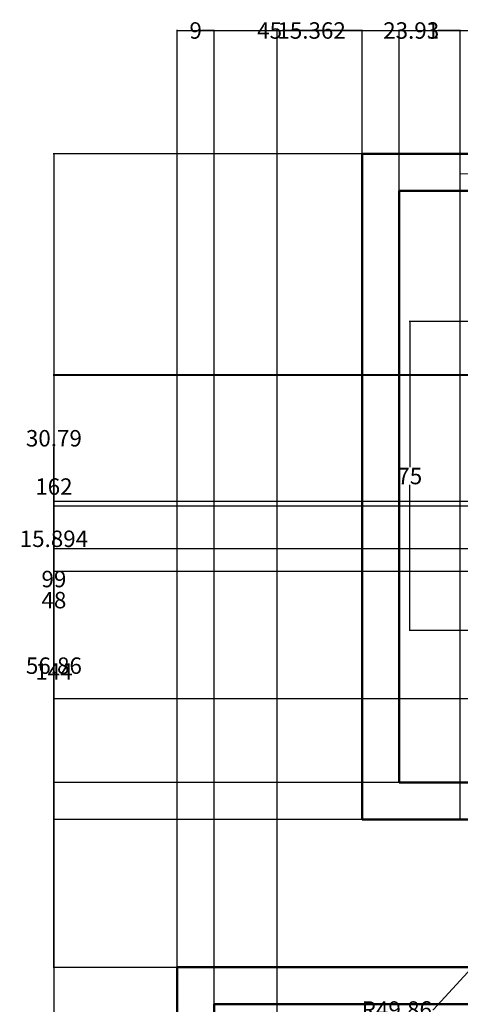
# Model space of a CAD drawing. Units: inches. Extents: x 1454 to 2136, y 626 to 1213.
# Tile 5 of 23: x 1454 to 1561, y 973 to 1213. Entities that reach past the tile are written whole.
import ezdxf

# ---------------------------------------------------------------- set-up
doc = ezdxf.new("R2010")
doc.units = ezdxf.units.IN
doc.header["$MEASUREMENT"] = 0
for name, color, linetype, lineweight in [('A-ANNO-DIMS', 2, 'Continuous', 18), ('A-FURN-PATT', 252, 'Continuous', 13), ('A-GLAZ', 4, 'Continuous', 18), ('A-WALL', 7, 'Continuous', 50)]:
    doc.layers.add(name, color=color, linetype=linetype, lineweight=lineweight)
doc.styles.get("Standard").update_dxf_attribs({"font": 'arial.ttf'})
doc.dimstyles.get("Standard").update_dxf_attribs({"dimtxt": 4, "dimasz": 0.18, "dimexe": 0.18, "dimexo": 0.0625, "dimgap": 0.09, "dimtad": 0, "dimtih": 1, "dimtoh": 1, "dimdec": 0, "dimrnd": 6, "dimzin": 0, "dimdsep": 46, "dimlunit": 3, "dimtxsty": 'Standard', "dimcen": 0.09, "dimadec": 0, "dimazin": 0, "dimtfac": 1, "dimtdec": 0, "dimtofl": 0, "dimtmove": 0, "dimatfit": 3, "dimfxl": 1, "dimtolj": 1, "dimtzin": 0, "dimarcsym": 0})

# ---------------------------------------------------------------- blocks, each defined once
blk = doc.blocks.new('WIN-34_84')
blk.add_line((34.84, 4.31), (0, 4.31))
blk.add_lwpolyline([(34.84, 0), (0, 0), (0, 9), (34.84, 9)], close=True)
blk = doc.blocks.new('*D24')
at = {"layer": 'A-ANNO-DIMS', "color": 0, "lineweight": -2, "transparency": 16777216}
for p, q in [((1571.61, 1139.47), (1548.99, 1139.47)), ((1549.17, 1139.29), (1549.17, 1103.97)), ((1549.17, 1064.4), (1549.17, 1099.72)), ((1571.61, 1064.22), (1548.99, 1064.22))]:
    blk.add_line(p, q, dxfattribs=at)
at = {"layer": 'A-ANNO-DIMS', "color": 0, "transparency": 16777216}
for points in [[(1549.14, 1139.29), (1549.2, 1139.29), (1549.17, 1139.47)], [(1549.14, 1064.4), (1549.2, 1064.4), (1549.17, 1064.22)]]:
    blk.add_solid(points, dxfattribs=at)
at = {"layer": 'Defpoints', "color": 0, "transparency": 16777216}
for p in [(1549.17, 1139.47), (1571.67, 1139.47), (1571.67, 1064.22)]:
    blk.add_point(p, dxfattribs=at)
at = {"layer": 'A-ANNO-DIMS', "color": 0, "transparency": 16777216, "insert": (1549.17, 1101.85), "char_height": 4, "attachment_point": 5}
blk.add_mtext('\\A1;75', dxfattribs=at)
blk = doc.blocks.new('*D28')
at = {"layer": 'A-ANNO-DIMS', "color": 0, "lineweight": -2, "transparency": 16777216}
for p, q in [((1537.49, 1180.28), (1462.37, 1180.28)), ((1462.55, 1180.1), (1462.55, 921.41)), ((1462.55, 658.46), (1462.55, 917.15)), ((1492.49, 658.28), (1462.37, 658.28))]:
    blk.add_line(p, q, dxfattribs=at)
at = {"layer": 'A-ANNO-DIMS', "color": 0, "transparency": 16777216}
for points in [[(1462.52, 1180.1), (1462.58, 1180.1), (1462.55, 1180.28)], [(1462.52, 658.46), (1462.58, 658.46), (1462.55, 658.28)]]:
    blk.add_solid(points, dxfattribs=at)
at = {"layer": 'Defpoints', "color": 0, "transparency": 16777216}
for p in [(1462.55, 1180.28), (1537.56, 1180.28), (1492.56, 658.28)]:
    blk.add_point(p, dxfattribs=at)
at = {"layer": 'A-ANNO-DIMS', "color": 0, "transparency": 16777216, "insert": (1462.55, 919.28), "char_height": 4, "attachment_point": 5}
blk.add_mtext('\\A1;522', dxfattribs=at)
blk = doc.blocks.new('*D29')
at = {"layer": 'A-ANNO-DIMS', "color": 0, "lineweight": -2, "transparency": 16777216}
for p, q in [((1546.56, 1171.34), (1546.56, 1210.46)), ((1546.74, 1210.28), (1644.02, 1210.28)), ((1750.38, 1210.28), (1653.09, 1210.28)), ((1750.56, 1171.34), (1750.56, 1210.46))]:
    blk.add_line(p, q, dxfattribs=at)
at = {"layer": 'A-ANNO-DIMS', "color": 0, "transparency": 16777216}
for points in [[(1546.74, 1210.31), (1546.74, 1210.25), (1546.56, 1210.28)], [(1750.38, 1210.31), (1750.38, 1210.25), (1750.56, 1210.28)]]:
    blk.add_solid(points, dxfattribs=at)
at = {"layer": 'Defpoints', "color": 0, "transparency": 16777216}
for p in [(1750.56, 1210.28), (1546.56, 1171.28), (1750.56, 1171.28)]:
    blk.add_point(p, dxfattribs=at)
at = {"layer": 'A-ANNO-DIMS', "color": 0, "transparency": 16777216, "insert": (1648.56, 1210.28), "char_height": 4, "attachment_point": 5}
blk.add_mtext('\\A1;204', dxfattribs=at)
blk = doc.blocks.new('*D30')
at = {"layer": 'A-ANNO-DIMS', "color": 0, "lineweight": -2, "transparency": 16777216}
for p, q in [((1537.49, 1180.28), (1462.37, 1180.28)), ((1462.55, 1180.1), (1462.55, 1101.41)), ((1462.55, 1018.46), (1462.55, 1097.15)), ((1537.49, 1018.28), (1462.37, 1018.28))]:
    blk.add_line(p, q, dxfattribs=at)
at = {"layer": 'A-ANNO-DIMS', "color": 0, "transparency": 16777216}
for points in [[(1462.52, 1180.1), (1462.58, 1180.1), (1462.55, 1180.28)], [(1462.52, 1018.46), (1462.58, 1018.46), (1462.55, 1018.28)]]:
    blk.add_solid(points, dxfattribs=at)
at = {"layer": 'Defpoints', "color": 0, "transparency": 16777216}
for p in [(1462.55, 1180.28), (1537.56, 1180.28), (1537.56, 1018.28)]:
    blk.add_point(p, dxfattribs=at)
at = {"layer": 'A-ANNO-DIMS', "color": 0, "transparency": 16777216, "insert": (1462.55, 1099.28), "char_height": 4, "attachment_point": 5}
blk.add_mtext('\\A1;162', dxfattribs=at)
blk = doc.blocks.new('*D33')
at = {"layer": 'A-ANNO-DIMS', "color": 0, "lineweight": -2, "transparency": 16777216}
for p, q in [((2032.49, 1126.28), (1462.37, 1126.28)), ((1462.55, 1126.1), (1462.55, 1056.38)), ((1462.55, 982.46), (1462.55, 1052.18)), ((2032.49, 982.28), (1462.37, 982.28))]:
    blk.add_line(p, q, dxfattribs=at)
at = {"layer": 'A-ANNO-DIMS', "color": 0, "transparency": 16777216}
for points in [[(1462.52, 1126.1), (1462.58, 1126.1), (1462.55, 1126.28)], [(1462.52, 982.46), (1462.58, 982.46), (1462.55, 982.28)]]:
    blk.add_solid(points, dxfattribs=at)
at = {"layer": 'Defpoints', "color": 0, "transparency": 16777216}
for p in [(1462.55, 1126.28), (2032.56, 1126.28), (2032.56, 982.28)]:
    blk.add_point(p, dxfattribs=at)
at = {"layer": 'A-ANNO-DIMS', "color": 0, "transparency": 16777216, "insert": (1462.55, 1054.28), "char_height": 4, "attachment_point": 5}
blk.add_mtext('\\A1;144', dxfattribs=at)
blk = doc.blocks.new('*D39')
at = {"layer": 'A-ANNO-DIMS', "color": 0, "lineweight": -2, "transparency": 16777216}
for p, q in [((1492.56, 982.34), (1492.56, 1210.46)), ((1492.74, 1210.28), (1512.01, 1210.28)), ((1537.38, 1210.28), (1518.11, 1210.28)), ((1537.56, 1018.34), (1537.56, 1210.46))]:
    blk.add_line(p, q, dxfattribs=at)
at = {"layer": 'A-ANNO-DIMS', "color": 0, "transparency": 16777216}
for points in [[(1492.74, 1210.31), (1492.74, 1210.25), (1492.56, 1210.28)], [(1537.38, 1210.31), (1537.38, 1210.25), (1537.56, 1210.28)]]:
    blk.add_solid(points, dxfattribs=at)
at = {"layer": 'Defpoints', "color": 0, "transparency": 16777216}
for p in [(1537.56, 1210.28), (1537.56, 1018.28), (1492.56, 982.28)]:
    blk.add_point(p, dxfattribs=at)
at = {"layer": 'A-ANNO-DIMS', "color": 0, "transparency": 16777216, "insert": (1515.06, 1210.28), "char_height": 4, "attachment_point": 5}
blk.add_mtext('\\A1;45', dxfattribs=at)
blk = doc.blocks.new('*D40')
at = {"layer": 'A-ANNO-DIMS', "color": 0, "lineweight": -2, "transparency": 16777216}
for p, q in [((1501.56, 877.34), (1501.56, 1210.46)), ((1501.74, 1210.28), (1569.24, 1210.28)), ((1645.38, 1210.28), (1577.87, 1210.28)), ((1645.56, 877.34), (1645.56, 1210.46))]:
    blk.add_line(p, q, dxfattribs=at)
at = {"layer": 'A-ANNO-DIMS', "color": 0, "transparency": 16777216}
for points in [[(1501.74, 1210.31), (1501.74, 1210.25), (1501.56, 1210.28)], [(1645.38, 1210.31), (1645.38, 1210.25), (1645.56, 1210.28)]]:
    blk.add_solid(points, dxfattribs=at)
at = {"layer": 'Defpoints', "color": 0, "transparency": 16777216}
for p in [(1645.56, 1210.28), (1501.56, 877.28), (1645.56, 877.28)]:
    blk.add_point(p, dxfattribs=at)
at = {"layer": 'A-ANNO-DIMS', "color": 0, "transparency": 16777216, "insert": (1573.56, 1210.28), "char_height": 4, "attachment_point": 5}
blk.add_mtext('\\A1;144', dxfattribs=at)
blk = doc.blocks.new('*D49')
at = {"layer": 'A-ANNO-DIMS', "color": 0, "lineweight": -2, "transparency": 16777216}
for p, q in [((1537.56, 1180.34), (1537.56, 1210.46)), ((1537.74, 1210.28), (1543.02, 1210.28)), ((1561.28, 1210.28), (1556, 1210.28)), ((1561.46, 1180.17), (1561.46, 1210.46))]:
    blk.add_line(p, q, dxfattribs=at)
at = {"layer": 'A-ANNO-DIMS', "color": 0, "transparency": 16777216}
for points in [[(1537.74, 1210.31), (1537.74, 1210.25), (1537.56, 1210.28)], [(1561.28, 1210.31), (1561.28, 1210.25), (1561.46, 1210.28)]]:
    blk.add_solid(points, dxfattribs=at)
at = {"layer": 'Defpoints', "color": 0, "transparency": 16777216}
for p in [(1561.46, 1210.28), (1537.56, 1180.28), (1561.46, 1180.1)]:
    blk.add_point(p, dxfattribs=at)
at = {"layer": 'A-ANNO-DIMS', "color": 0, "transparency": 16777216, "insert": (1549.51, 1210.28), "char_height": 4, "attachment_point": 5}
blk.add_mtext('\\A1;23.91', dxfattribs=at)
blk = doc.blocks.new('*D54')
at = {"layer": 'A-ANNO-DIMS', "color": 0, "lineweight": -2, "transparency": 16777216}
for p, q in [((1879.49, 1126.28), (1462.37, 1126.28)), ((1462.55, 1126.1), (1462.55, 1078.91)), ((1462.55, 1027.46), (1462.55, 1074.65)), ((1879.49, 1027.28), (1462.37, 1027.28))]:
    blk.add_line(p, q, dxfattribs=at)
at = {"layer": 'A-ANNO-DIMS', "color": 0, "transparency": 16777216}
for points in [[(1462.52, 1126.1), (1462.58, 1126.1), (1462.55, 1126.28)], [(1462.52, 1027.46), (1462.58, 1027.46), (1462.55, 1027.28)]]:
    blk.add_solid(points, dxfattribs=at)
at = {"layer": 'Defpoints', "color": 0, "transparency": 16777216}
for p in [(1879.56, 1126.28), (1462.55, 1027.28), (1879.56, 1027.28)]:
    blk.add_point(p, dxfattribs=at)
at = {"layer": 'A-ANNO-DIMS', "color": 0, "transparency": 16777216, "insert": (1462.55, 1076.78), "char_height": 4, "attachment_point": 5}
blk.add_mtext('\\A1;99', dxfattribs=at)
blk = doc.blocks.new('*D55')
at = {"layer": 'A-ANNO-DIMS', "color": 0, "lineweight": -2, "transparency": 16777216}
for p, q in [((1537.56, 1018.34), (1537.56, 1210.46)), ((1537.74, 1210.28), (1542.65, 1210.28)), ((1561.3, 1210.28), (1556.39, 1210.28)), ((1561.48, 1018.34), (1561.48, 1210.46))]:
    blk.add_line(p, q, dxfattribs=at)
at = {"layer": 'A-ANNO-DIMS', "color": 0, "transparency": 16777216}
for points in [[(1537.74, 1210.31), (1537.74, 1210.25), (1537.56, 1210.28)], [(1561.3, 1210.31), (1561.3, 1210.25), (1561.48, 1210.28)]]:
    blk.add_solid(points, dxfattribs=at)
at = {"layer": 'Defpoints', "color": 0, "transparency": 16777216}
for p in [(1561.48, 1210.28), (1537.56, 1018.28), (1561.48, 1018.28)]:
    blk.add_point(p, dxfattribs=at)
at = {"layer": 'A-ANNO-DIMS', "color": 0, "transparency": 16777216, "insert": (1549.52, 1210.28), "char_height": 4, "attachment_point": 5}
blk.add_mtext('\\A1;23.93', dxfattribs=at)
blk = doc.blocks.new('*D70')
at = {"layer": 'A-ANNO-DIMS', "color": 0, "lineweight": -2, "transparency": 16777216}
for p, q in [((1811.17, 1094.52), (1462.37, 1094.52)), ((1462.55, 1094.34), (1462.55, 1088.71)), ((1462.55, 1078.81), (1462.55, 1084.45)), ((1811.17, 1078.63), (1462.37, 1078.63))]:
    blk.add_line(p, q, dxfattribs=at)
at = {"layer": 'A-ANNO-DIMS', "color": 0, "transparency": 16777216}
for points in [[(1462.52, 1094.34), (1462.58, 1094.34), (1462.55, 1094.52)], [(1462.52, 1078.81), (1462.58, 1078.81), (1462.55, 1078.63)]]:
    blk.add_solid(points, dxfattribs=at)
at = {"layer": 'Defpoints', "color": 0, "transparency": 16777216}
for p in [(1462.55, 1094.52), (1811.23, 1094.52), (1811.23, 1078.63)]:
    blk.add_point(p, dxfattribs=at)
at = {"layer": 'A-ANNO-DIMS', "color": 0, "transparency": 16777216, "insert": (1462.55, 1086.58), "char_height": 4, "attachment_point": 5}
blk.add_mtext('\\A1;15.894', dxfattribs=at)
blk = doc.blocks.new('*D73')
at = {"layer": 'A-ANNO-DIMS', "color": 0, "lineweight": -2, "transparency": 16777216}
for p, q in [((1985.1, 1126.44), (1462.37, 1126.44)), ((1462.55, 1126.26), (1462.55, 1113.18)), ((1462.55, 1095.83), (1462.55, 1108.91)), ((1966.64, 1095.65), (1462.37, 1095.65))]:
    blk.add_line(p, q, dxfattribs=at)
at = {"layer": 'A-ANNO-DIMS', "color": 0, "transparency": 16777216}
for points in [[(1462.52, 1126.26), (1462.58, 1126.26), (1462.55, 1126.44)], [(1462.52, 1095.83), (1462.58, 1095.83), (1462.55, 1095.65)]]:
    blk.add_solid(points, dxfattribs=at)
at = {"layer": 'Defpoints', "color": 0, "transparency": 16777216}
for p in [(1985.16, 1126.44), (1462.55, 1095.65), (1966.71, 1095.65)]:
    blk.add_point(p, dxfattribs=at)
at = {"layer": 'A-ANNO-DIMS', "color": 0, "transparency": 16777216, "insert": (1462.55, 1111.04), "char_height": 4, "attachment_point": 5}
blk.add_mtext('\\A1;30.79', dxfattribs=at)
blk = doc.blocks.new('*D76')
at = {"layer": 'A-ANNO-DIMS', "color": 0, "lineweight": -2, "transparency": 16777216}
for p, q in [((1962.64, 1095.65), (1462.37, 1095.65)), ((1462.55, 1095.47), (1462.55, 1073.78)), ((1462.55, 1047.83), (1462.55, 1069.52)), ((1914.64, 1047.65), (1462.37, 1047.65))]:
    blk.add_line(p, q, dxfattribs=at)
at = {"layer": 'A-ANNO-DIMS', "color": 0, "transparency": 16777216}
for points in [[(1462.52, 1095.47), (1462.58, 1095.47), (1462.55, 1095.65)], [(1462.52, 1047.83), (1462.58, 1047.83), (1462.55, 1047.65)]]:
    blk.add_solid(points, dxfattribs=at)
at = {"layer": 'Defpoints', "color": 0, "transparency": 16777216}
for p in [(1962.71, 1095.65), (1462.55, 1047.65), (1914.71, 1047.65)]:
    blk.add_point(p, dxfattribs=at)
at = {"layer": 'A-ANNO-DIMS', "color": 0, "transparency": 16777216, "insert": (1462.55, 1071.65), "char_height": 4, "attachment_point": 5}
blk.add_mtext('\\A1;48', dxfattribs=at)
blk = doc.blocks.new('*D79')
at = {"layer": 'A-ANNO-DIMS', "color": 0, "lineweight": -2, "transparency": 16777216}
for p, q in [((1501.56, 973.34), (1501.56, 1210.46)), ((1501.74, 1210.28), (1516.74, 1210.28)), ((1516.92, 962.3), (1516.92, 1210.46)), ((1516.92, 1210.28), (1517.1, 1210.28))]:
    blk.add_line(p, q, dxfattribs=at)
at = {"layer": 'A-ANNO-DIMS', "color": 0, "transparency": 16777216}
for points in [[(1501.74, 1210.31), (1501.74, 1210.25), (1501.56, 1210.28)], [(1516.74, 1210.31), (1516.74, 1210.25), (1516.92, 1210.28)]]:
    blk.add_solid(points, dxfattribs=at)
at = {"layer": 'Defpoints', "color": 0, "transparency": 16777216}
for p in [(1516.92, 1210.28), (1501.56, 973.28), (1516.92, 962.24)]:
    blk.add_point(p, dxfattribs=at)
at = {"layer": 'A-ANNO-DIMS', "color": 0, "transparency": 16777216, "insert": (1525.28, 1210.28), "char_height": 4, "attachment_point": 5}
blk.add_mtext('\\A1;15.362', dxfattribs=at)
blk = doc.blocks.new('*D82')
at = {"layer": 'A-ANNO-DIMS', "color": 0, "lineweight": -2, "transparency": 16777216}
for p, q in [((1697.82, 1084.13), (1462.37, 1084.13)), ((1462.55, 1083.95), (1462.55, 1057.83)), ((1462.55, 1027.45), (1462.55, 1053.57)), ((1704.25, 1027.27), (1462.37, 1027.27))]:
    blk.add_line(p, q, dxfattribs=at)
at = {"layer": 'A-ANNO-DIMS', "color": 0, "transparency": 16777216}
for points in [[(1462.52, 1083.95), (1462.58, 1083.95), (1462.55, 1084.13)], [(1462.52, 1027.45), (1462.58, 1027.45), (1462.55, 1027.27)]]:
    blk.add_solid(points, dxfattribs=at)
at = {"layer": 'Defpoints', "color": 0, "transparency": 16777216}
for p in [(1462.55, 1084.13), (1697.88, 1084.13), (1704.31, 1027.27)]:
    blk.add_point(p, dxfattribs=at)
at = {"layer": 'A-ANNO-DIMS', "color": 0, "transparency": 16777216, "insert": (1462.55, 1055.7), "char_height": 4, "attachment_point": 5}
blk.add_mtext('\\A1;56.86', dxfattribs=at)
blk = doc.blocks.new('*D88')
at = {"layer": 'A-ANNO-DIMS', "color": 0, "lineweight": -2, "transparency": 16777216}
for p, q in [((1492.56, 658.34), (1492.56, 1210.46)), ((1492.74, 1210.28), (1495.65, 1210.28)), ((1501.38, 1210.28), (1498.46, 1210.28)), ((1501.56, 667.34), (1501.56, 1210.46))]:
    blk.add_line(p, q, dxfattribs=at)
at = {"layer": 'A-ANNO-DIMS', "color": 0, "transparency": 16777216}
for points in [[(1492.74, 1210.31), (1492.74, 1210.25), (1492.56, 1210.28)], [(1501.38, 1210.31), (1501.38, 1210.25), (1501.56, 1210.28)]]:
    blk.add_solid(points, dxfattribs=at)
at = {"layer": 'Defpoints', "color": 0, "transparency": 16777216}
for p in [(1501.56, 1210.28), (1501.56, 667.28), (1492.56, 658.28)]:
    blk.add_point(p, dxfattribs=at)
at = {"layer": 'A-ANNO-DIMS', "color": 0, "transparency": 16777216, "insert": (1497.06, 1210.28), "char_height": 4, "attachment_point": 5}
blk.add_mtext('\\A1;9', dxfattribs=at)
blk = doc.blocks.new('*D92')
at = {"layer": 'A-ANNO-DIMS', "color": 0, "lineweight": -2, "transparency": 16777216}
for p, q in [((1608.77, 1030.83), (1608.95, 1030.83)), ((1608.86, 1030.74), (1608.86, 1030.92)), ((1554.95, 972.02), (1575.05, 993.94)), ((1554.77, 972.02), (1554.95, 972.02))]:
    blk.add_line(p, q, dxfattribs=at)
at = {"layer": 'A-ANNO-DIMS', "color": 0, "transparency": 16777216}
blk.add_solid([(1575.02, 993.96), (1575.07, 993.92), (1575.17, 994.07)], dxfattribs=at)
at = {"layer": 'Defpoints', "color": 0, "transparency": 16777216}
for p in [(1608.86, 1030.83), (1575.17, 994.07)]:
    blk.add_point(p, dxfattribs=at)
at = {"layer": 'A-ANNO-DIMS', "color": 0, "transparency": 16777216, "insert": (1546.02, 972.02), "char_height": 4, "attachment_point": 5}
blk.add_mtext('\\A1;R49.86', dxfattribs=at)

msp = doc.modelspace()

# ---------------------------------------------------------------- hatches: boundary and pattern name
at = {"layer": 'A-FURN-PATT'}
h = msp.add_hatch(dxfattribs=at)
h.set_pattern_fill('ESCHER', color=256)
h.paths.add_polyline_path([(1511.3761, 923.7174, 1), (1525.379, 923.7174, 1)])
h.paths.add_polyline_path([(1525.379, 816.0542, 1), (1511.3761, 816.0542, 1)])
h.paths.add_polyline_path([(1525.379, 712.7345, 1), (1511.3761, 712.7345, 1)])
h.paths.add_polyline_path([(2070.5057, 794.3402, 1), (2056.5027, 794.3402, 1)])
h.paths.add_polyline_path([(2005.868, 1014.5578, 1), (1991.8651, 1014.5578, 1)])
h.paths.add_polyline_path([(1994.0647, 1066.7584, 1), (2008.0677, 1066.7584, 1)])
h.paths.add_polyline_path([(1919.5492, 1065.3848, 1), (1933.5521, 1065.3848, 1)])
h.paths.add_polyline_path([(1936.8517, 1013.7336, 1), (1922.8488, 1013.7336, 1)])
h.paths.add_polyline_path([(1824.6062, 1109.1557, 1), (1838.6091, 1109.1557, 1)])

# ---------------------------------------------------------------- linework, layer by layer
at = {"layer": 'A-WALL'}
for p, q in [((1759.5563, 1180.2825), (1537.5563, 1180.2825)), ((1537.5563, 1180.2825), (1537.5563, 1018.2825)), ((1750.5563, 1171.2825), (1546.5563, 1171.2825)), ((1546.5563, 1171.2825), (1546.5563, 1027.2825)), ((1750.5563, 1027.2825), (1546.5563, 1027.2825)), ((1843.5563, 1018.2825), (1537.5563, 1018.2825)), ((1492.5563, 982.2825), (1492.5563, 700.2825)), ((1654.5563, 982.2825), (1492.5563, 982.2825)), ((1501.5563, 973.2825), (1501.5563, 877.2825)), ((1645.5563, 973.2825), (1501.5563, 973.2825))]:
    msp.add_line(p, q, dxfattribs=at)

# ---------------------------------------------------------------- block references
at = {"layer": 'A-GLAZ'}
msp.add_blockref('WIN-34_84', (1561.4646, 1171.1038), dxfattribs=at)

# ---------------------------------------------------------------- dimensions: what is measured, and where the dimension line sits
at = {"layer": 'A-ANNO-DIMS'}
for base, p1, p2, override, picture, middle in [((1537.5563, 1210.2845), (1492.5563, 982.2825), (1537.5563, 1018.2825), {"dimdec": 0, "dimlfac": 1, "dimrnd": 0, "dimzin": 0, "dimdsep": 46, "dimlunit": 2}, '*D39', (1515.0563, 1210.2845)), ((1501.5563, 1210.2845), (1492.5563, 658.2825), (1501.5563, 667.2825), {"dimdec": 0, "dimlfac": 1, "dimrnd": 0, "dimzin": 0, "dimdsep": 46, "dimlunit": 2}, '*D88', (1497.0563, 1210.2845)), ((1645.5563, 1210.2845), (1501.5563, 877.2825), (1645.5563, 877.2825), {"dimdec": 0, "dimlfac": 1, "dimrnd": 0, "dimzin": 0, "dimdsep": 46, "dimlunit": 2}, '*D40', (1573.5563, 1210.2845)), ((1516.9185, 1210.2845), (1501.5563, 973.2825), (1516.9185, 962.2419), {"dimdec": 3, "dimlfac": 1, "dimrnd": 0, "dimzin": 0, "dimdsep": 46, "dimlunit": 2}, '*D79', (1525.2826, 1210.2845)), ((1561.4646, 1210.2845), (1537.5563, 1180.2825), (1561.4646, 1180.1038), {"dimdec": 2, "dimlfac": 1, "dimrnd": 0, "dimzin": 0, "dimdsep": 46, "dimlunit": 2}, '*D49', (1549.5105, 1210.2845)), ((1561.4844, 1210.2845), (1537.5563, 1018.2825), (1561.4844, 1018.2825), {"dimdec": 2, "dimlfac": 1, "dimrnd": 0, "dimzin": 0, "dimdsep": 46, "dimlunit": 2}, '*D55', (1549.5203, 1210.2845)), ((1750.5563, 1210.2845), (1546.5563, 1171.2825), (1750.5563, 1171.2825), {"dimdec": 0, "dimlfac": 1, "dimrnd": 0, "dimzin": 0, "dimdsep": 46, "dimlunit": 2}, '*D29', (1648.5563, 1210.2845))]:
    dim = msp.add_linear_dim(base=base, p1=p1, p2=p2, dimstyle='Standard', override=override, dxfattribs=at)
    dim.commit()
    dim.dimension.update_dxf_attribs({"geometry": picture, "text_midpoint": middle})
for base, p1, p2, override, picture, middle in [((1462.5543, 1180.2825), (1492.5563, 658.2825), (1537.5563, 1180.2825), {"dimdec": 0, "dimlfac": 1, "dimrnd": 0, "dimzin": 0, "dimdsep": 46, "dimlunit": 2}, '*D28', (1462.5543, 919.2825)), ((1462.5543, 1180.2825), (1537.5563, 1018.2825), (1537.5563, 1180.2825), {"dimdec": 0, "dimlfac": 1, "dimrnd": 0, "dimzin": 0, "dimdsep": 46, "dimlunit": 2}, '*D30', (1462.5543, 1099.2825)), ((1549.1663, 1139.4691), (1571.674, 1064.221), (1571.674, 1139.4691), {"dimdec": 0, "dimlfac": 1, "dimrnd": 0, "dimzin": 0, "dimdsep": 46, "dimlunit": 2}, '*D24', (1549.1663, 1101.8451)), ((1462.5543, 1095.6495), (1985.1581, 1126.439), (1966.7068, 1095.6495), {"dimdec": 2, "dimlfac": 1, "dimrnd": 0, "dimzin": 0, "dimdsep": 46, "dimlunit": 2}, '*D73', (1462.5543, 1111.0443)), ((1462.5543, 1126.2825), (2032.5563, 982.2825), (2032.5563, 1126.2825), {"dimdec": 0, "dimlfac": 1, "dimrnd": 0, "dimzin": 0, "dimdsep": 46, "dimlunit": 2}, '*D33', (1462.5543, 1054.2825)), ((1462.5543, 1027.2825), (1879.5563, 1126.2825), (1879.5563, 1027.2825), {"dimdec": 0, "dimlfac": 1, "dimrnd": 0, "dimzin": 0, "dimdsep": 46, "dimlunit": 2}, '*D54', (1462.5543, 1076.7825)), ((1462.5543, 1047.6495), (1962.7068, 1095.6495), (1914.7068, 1047.6495), {"dimdec": 0, "dimlfac": 1, "dimrnd": 0, "dimzin": 0, "dimdsep": 46, "dimlunit": 2}, '*D76', (1462.5543, 1071.6495)), ((1462.5543, 1094.5248), (1811.2288, 1078.6305), (1811.2288, 1094.5248), {"dimdec": 3, "dimlfac": 1, "dimrnd": 0, "dimzin": 0, "dimdsep": 46, "dimlunit": 2}, '*D70', (1462.5543, 1086.5777)), ((1462.5543, 1084.1285), (1704.308, 1027.2667), (1697.8807, 1084.1285), {"dimdec": 2, "dimlfac": 1, "dimrnd": 0, "dimzin": 0, "dimdsep": 46, "dimlunit": 2}, '*D82', (1462.5543, 1055.6976))]:
    dim = msp.add_linear_dim(base=base, p1=p1, p2=p2, angle=90, dimstyle='Standard', override=override, dxfattribs=at)
    dim.commit()
    dim.dimension.update_dxf_attribs({"geometry": picture, "text_midpoint": middle})
dim = msp.add_radius_dim(center=(1608.86, 1030.8286), mpoint=(1575.1679, 994.0729), dimstyle='Standard', override={"dimdec": 2, "dimlfac": 1, "dimrnd": 0, "dimzin": 0, "dimdsep": 46, "dimlunit": 2}, dxfattribs=at)
dim.commit()
dim.dimension.update_dxf_attribs({"geometry": '*D92', "text_midpoint": (1546.0211, 972.0196), "dimtype": 164})

doc.saveas('drawing.dxf')
